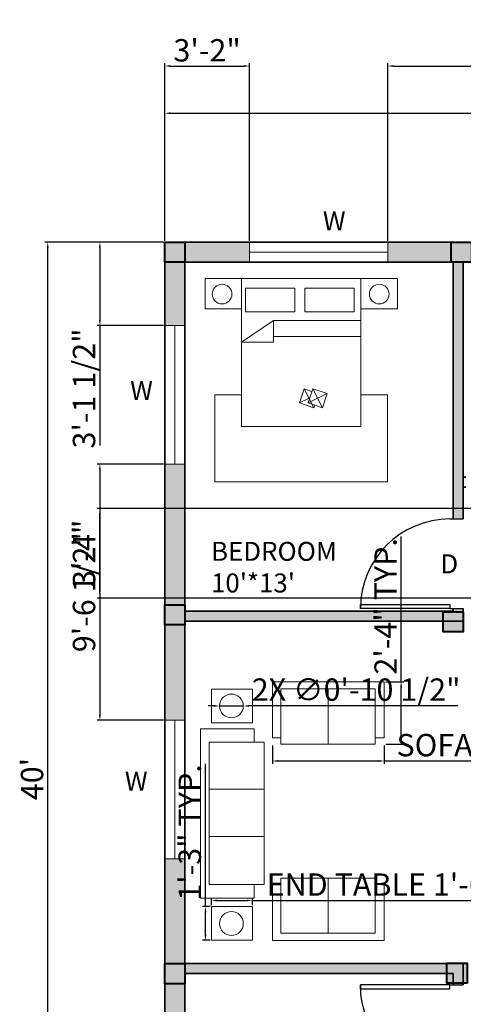
# Model space of a CAD drawing. Units: inches. Extents: x 1801 to 2333, y 2020 to 2714.
# Tile 2 of 4: x 1801 to 1999, y 2274 to 2714. Entities that reach past the tile are written whole.
import ezdxf

# ---------------------------------------------------------------- set-up
doc = ezdxf.new("R2010")
doc.units = ezdxf.units.IN
for name, color, linetype, lineweight in [('A-ANNO-DIMS', 2, 'Continuous', 18), ('A-ANNO-TEXT', 200, 'Continuous', 18), ('A-AREA-IDEN', 200, 'Continuous', 25), ('A-COLS', 7, 'Continuous', 40), ('A-COLS-PATT', 250, 'Continuous', 13), ('A-DOOR', 4, 'Continuous', 25), ('A-FURN', 8, 'Continuous', 18), ('A-WALL-PATT', 252, 'Continuous', 13), ('WALL', 150, 'Continuous', 35), ('WINDOW', 130, 'Continuous', 18)]:
    doc.layers.add(name, color=color, linetype=linetype, lineweight=lineweight)
doc.styles.get("Standard").update_dxf_attribs({"font": 'arial.ttf'})
doc.dimstyles.new('ISO-25', dxfattribs={"dimtxt": 10, "dimasz": 2.5, "dimexe": 1.25, "dimexo": 0.625, "dimtad": 1, "dimdec": 0, "dimlunit": 4, "dimtxsty": 'Standard', "dimcen": 2.5, "dimadec": 0, "dimazin": 0, "dimtfac": 1, "dimtdec": 0, "dimtmove": 0, "dimatfit": 3, "dimfxl": 1, "dimarcsym": 0})

# ---------------------------------------------------------------- blocks, each defined once
blk = doc.blocks.new('*U2')
for p, q in [((0, 0), (0, -6)), ((40, 0), (40, -6))]:
    blk.add_line(p, q)
blk.add_lwpolyline([(0, 0), (0, 40), (1.75, 40), (1.75, 0)], close=True)
blk.add_arc((0, 0), 40, 0, 90)
blk = doc.blocks.new('*D7')
at = {"layer": 'A-ANNO-DIMS', "color": 0, "lineweight": -2, "transparency": 16777216}
for p, q in [((1865.69, 2614.97), (1865.69, 2673.24)), ((1868.19, 2671.99), (2247.19, 2671.99)), ((2249.69, 2614.97), (2249.69, 2673.24))]:
    blk.add_line(p, q, dxfattribs=at)
at = {"layer": 'A-ANNO-DIMS', "color": 0, "transparency": 16777216}
for points in [[(1868.19, 2672.4), (1868.19, 2671.57), (1865.69, 2671.99)], [(2247.19, 2672.4), (2247.19, 2671.57), (2249.69, 2671.99)]]:
    blk.add_solid(points, dxfattribs=at)
at = {"layer": 'Defpoints', "color": 0, "transparency": 16777216}
for p in [(2249.69, 2671.99), (1865.69, 2614.35), (2249.69, 2614.35)]:
    blk.add_point(p, dxfattribs=at)
at = {"layer": 'A-ANNO-DIMS', "color": 0, "transparency": 16777216, "insert": (2057.69, 2677.72), "char_height": 10, "attachment_point": 5}
blk.add_mtext("32'", dxfattribs=at)
blk = doc.blocks.new('*D8')
at = {"layer": 'A-ANNO-DIMS', "color": 0, "lineweight": -2, "transparency": 16777216}
for p, q in [((1865.06, 2614.35), (1812.13, 2614.35)), ((1813.38, 2136.85), (1813.38, 2611.85)), ((1865.06, 2134.35), (1812.13, 2134.35))]:
    blk.add_line(p, q, dxfattribs=at)
at = {"layer": 'A-ANNO-DIMS', "color": 0, "transparency": 16777216}
for points in [[(1812.96, 2611.85), (1813.79, 2611.85), (1813.38, 2614.35)], [(1812.96, 2136.85), (1813.79, 2136.85), (1813.38, 2134.35)]]:
    blk.add_solid(points, dxfattribs=at)
at = {"layer": 'Defpoints', "color": 0, "transparency": 16777216}
for p in [(1813.38, 2614.35), (1865.69, 2614.35), (1865.69, 2134.35)]:
    blk.add_point(p, dxfattribs=at)
at = {"layer": 'A-ANNO-DIMS', "color": 0, "transparency": 16777216, "insert": (1807.65, 2374.35), "char_height": 10, "attachment_point": 5, "rotation": 90}
blk.add_mtext("40'", dxfattribs=at)
blk = doc.blocks.new('BED-DOUBLE-WITH-NIGHTSTANDS')
for p, q in [((30.54, 72.05), (16.34, 62.37)), ((69.61, 72.05), (30.54, 72.05)), ((30.54, 62.37), (30.54, 72.05)), ((16.34, 62.37), (30.54, 62.37)), ((30.54, 64.89), (69.61, 64.89)), ((44.26, 41.5), (48.62, 33.08)), ((48.1, 41.5), (52.46, 33.08)), ((16.34, 38.79), (4.34, 38.79)), ((4.34, 38.79), (4.34, 0)), ((42.19, 35.19), (46.77, 37.46)), ((46.03, 35.19), (54.53, 39.39)), ((69.61, 38.79), (81.61, 38.79)), ((81.61, 38.79), (81.61, 0)), ((4.34, 0), (81.61, 0))]:
    blk.add_line(p, q)
for points in [[(0, 90.88), (16.34, 90.88), (16.34, 77.31), (0, 77.31)], [(16.34, 90.88), (69.61, 90.88), (69.61, 24.72), (16.34, 24.72)], [(69.61, 90.88), (85.96, 90.88), (85.96, 77.31), (69.61, 77.31)], [(18.06, 86.51), (40.1, 86.51), (40.1, 75.9), (18.06, 75.9)], [(44.61, 86.51), (66.65, 86.51), (66.65, 75.9), (44.61, 75.9)], [(46.03, 35.19), (48.1, 41.5), (54.53, 39.39), (52.46, 33.08)]]:
    blk.add_lwpolyline(points, close=True)
blk.add_lwpolyline([(48.99, 34.22), (48.62, 33.08), (42.19, 35.19), (44.26, 41.5), (47.73, 40.36)])
for centre in [(7.61, 83.86), (77.85, 83.86)]:
    blk.add_circle(centre, 4.4)
blk = doc.blocks.new('SOFA-TWO-SEAT')
for p, q in [((50.06, 27.92), (0, 27.92)), ((0, 27.92), (0, 2.87)), ((50.06, 2.87), (50.06, 27.92)), ((3.85, 24.67), (3.85, 0)), ((24.92, 24.67), (24.92, 0)), ((0, 2.87), (3.85, 2.87)), ((45.99, 2.87), (50.06, 2.87))]:
    blk.add_line(p, q)
blk.add_lwpolyline([(3.85, 0), (45.99, 0), (45.99, 24.67), (3.85, 24.67)])
blk = doc.blocks.new('TABLE-END-WITH-LAMP')
blk.add_lwpolyline([(0, 15.04), (18.33, 15.04), (18.33, 0), (0, 0)], close=True)
blk.add_circle((8.87, 7.48), 5.32)
blk = doc.blocks.new('WIN-STANDARD')
blk.add_line((0, 4.5), (61.87, 4.5))
blk.add_lwpolyline([(0, 9), (61.87, 9), (61.87, 0), (0, 0)], close=True)
blk = doc.blocks.new('COLUMN-9X9')
blk.add_lwpolyline([(0, 9), (9, 9), (9, 0), (0, 0)], close=True)
blk = doc.blocks.new('*D26')
at = {"layer": 'A-ANNO-DIMS', "color": 0, "lineweight": -2, "transparency": 16777216}
for p, q in [((1913.81, 2389.31), (1913.81, 2381.17)), ((1963.87, 2389.31), (1963.87, 2381.17)), ((1916.31, 2382.42), (1961.37, 2382.42)), ((1963.87, 2382.42), (2070.44, 2382.42))]:
    blk.add_line(p, q, dxfattribs=at)
at = {"layer": 'A-ANNO-DIMS', "color": 0, "transparency": 16777216}
for points in [[(1916.31, 2382.84), (1916.31, 2382.01), (1913.81, 2382.42)], [(1961.37, 2382.84), (1961.37, 2382.01), (1963.87, 2382.42)]]:
    blk.add_solid(points, dxfattribs=at)
at = {"layer": 'Defpoints', "color": 0, "transparency": 16777216}
for p in [(1913.81, 2389.93), (1963.87, 2389.93), (1963.87, 2382.42)]:
    blk.add_point(p, dxfattribs=at)
at = {"layer": 'A-ANNO-DIMS', "color": 0, "transparency": 16777216, "insert": (2018.41, 2388.22), "char_height": 10, "attachment_point": 5}
blk.add_mtext('SOFA 4\'-2" TYP.', dxfattribs=at)
blk = doc.blocks.new('*D27')
at = {"layer": 'A-ANNO-DIMS', "color": 0, "lineweight": -2, "transparency": 16777216}
for p, q in [((1971.38, 2417.85), (1971.38, 2482.73)), ((1964.49, 2417.85), (1972.63, 2417.85)), ((1971.38, 2392.43), (1971.38, 2415.35)), ((1964.49, 2389.93), (1972.63, 2389.93))]:
    blk.add_line(p, q, dxfattribs=at)
at = {"layer": 'A-ANNO-DIMS', "color": 0, "transparency": 16777216}
for points in [[(1970.96, 2415.35), (1971.79, 2415.35), (1971.38, 2417.85)], [(1970.96, 2392.43), (1971.79, 2392.43), (1971.38, 2389.93)]]:
    blk.add_solid(points, dxfattribs=at)
at = {"layer": 'Defpoints', "color": 0, "transparency": 16777216}
for p in [(1963.87, 2417.85), (1971.38, 2417.85), (1963.87, 2389.93)]:
    blk.add_point(p, dxfattribs=at)
at = {"layer": 'A-ANNO-DIMS', "color": 0, "transparency": 16777216, "insert": (1965.73, 2451.54), "char_height": 10, "attachment_point": 5, "rotation": 90}
blk.add_mtext('2\'-4" TYP.', dxfattribs=at)
blk = doc.blocks.new('*D28')
at = {"layer": 'A-ANNO-DIMS', "color": 0, "lineweight": -2, "transparency": 16777216}
for p, q in [((1886.64, 2317.95), (1886.64, 2321.32)), ((1889.14, 2320.07), (1902.46, 2320.07)), ((1904.96, 2317.95), (1904.96, 2321.32)), ((1904.96, 2320.07), (2073.96, 2320.07))]:
    blk.add_line(p, q, dxfattribs=at)
at = {"layer": 'A-ANNO-DIMS', "color": 0, "transparency": 16777216}
for points in [[(1889.14, 2320.49), (1889.14, 2319.65), (1886.64, 2320.07)], [(1902.46, 2320.49), (1902.46, 2319.65), (1904.96, 2320.07)]]:
    blk.add_solid(points, dxfattribs=at)
at = {"layer": 'Defpoints', "color": 0, "transparency": 16777216}
for p in [(1904.96, 2320.07), (1886.64, 2317.32), (1904.96, 2317.32)]:
    blk.add_point(p, dxfattribs=at)
at = {"layer": 'A-ANNO-DIMS', "color": 0, "transparency": 16777216, "insert": (1990.71, 2325.87), "char_height": 10, "attachment_point": 5}
blk.add_mtext('END TABLE 1\'-6 1/2" TYP.', dxfattribs=at)
blk = doc.blocks.new('*D29')
at = {"layer": 'A-ANNO-DIMS', "color": 0, "lineweight": -2, "transparency": 16777216}
for p, q in [((1883.89, 2317.32), (1883.89, 2381.09)), ((1886.01, 2317.32), (1882.64, 2317.32)), ((1883.89, 2304.78), (1883.89, 2314.82)), ((1886.01, 2302.28), (1882.64, 2302.28))]:
    blk.add_line(p, q, dxfattribs=at)
at = {"layer": 'A-ANNO-DIMS', "color": 0, "transparency": 16777216}
for points in [[(1883.47, 2314.82), (1884.3, 2314.82), (1883.89, 2317.32)], [(1883.47, 2304.78), (1884.3, 2304.78), (1883.89, 2302.28)]]:
    blk.add_solid(points, dxfattribs=at)
at = {"layer": 'Defpoints', "color": 0, "transparency": 16777216}
for p in [(1883.89, 2317.32), (1886.64, 2317.32), (1886.64, 2302.28)]:
    blk.add_point(p, dxfattribs=at)
at = {"layer": 'A-ANNO-DIMS', "color": 0, "transparency": 16777216, "insert": (1878.15, 2350.45), "char_height": 10, "attachment_point": 5, "rotation": 90}
blk.add_mtext('1\'-3" TYP.', dxfattribs=at)
blk = doc.blocks.new('*D30')
at = {"layer": 'A-ANNO-DIMS', "color": 0, "lineweight": -2, "transparency": 16777216}
for p, q in [((1865.69, 2614.97), (1865.69, 2694.33)), ((1903.59, 2614.97), (1903.59, 2694.33)), ((1868.19, 2693.08), (1901.09, 2693.08))]:
    blk.add_line(p, q, dxfattribs=at)
at = {"layer": 'A-ANNO-DIMS', "color": 0, "transparency": 16777216}
for points in [[(1868.19, 2693.5), (1868.19, 2692.66), (1865.69, 2693.08)], [(1901.09, 2693.5), (1901.09, 2692.66), (1903.59, 2693.08)]]:
    blk.add_solid(points, dxfattribs=at)
at = {"layer": 'Defpoints', "color": 0, "transparency": 16777216}
for p in [(1903.59, 2693.08), (1865.69, 2614.35), (1903.59, 2614.35)]:
    blk.add_point(p, dxfattribs=at)
at = {"layer": 'A-ANNO-DIMS', "color": 0, "transparency": 16777216, "insert": (1884.64, 2698.81), "char_height": 10, "attachment_point": 5}
blk.add_mtext('3\'-2"', dxfattribs=at)
blk = doc.blocks.new('*D31')
at = {"layer": 'A-ANNO-DIMS', "color": 0, "lineweight": -2, "transparency": 16777216}
for p, q in [((1965.46, 2614.97), (1965.46, 2694.33)), ((2008.88, 2614.97), (2008.88, 2694.33)), ((1967.96, 2693.08), (2006.38, 2693.08)), ((2008.88, 2693.08), (2062.5, 2693.08))]:
    blk.add_line(p, q, dxfattribs=at)
at = {"layer": 'A-ANNO-DIMS', "color": 0, "transparency": 16777216}
for points in [[(1967.96, 2693.5), (1967.96, 2692.66), (1965.46, 2693.08)], [(2006.38, 2693.5), (2006.38, 2692.66), (2008.88, 2693.08)]]:
    blk.add_solid(points, dxfattribs=at)
at = {"layer": 'Defpoints', "color": 0, "transparency": 16777216}
for p in [(2008.88, 2693.08), (1965.46, 2614.35), (2008.88, 2614.35)]:
    blk.add_point(p, dxfattribs=at)
at = {"layer": 'A-ANNO-DIMS', "color": 0, "transparency": 16777216, "insert": (2036.94, 2698.88), "char_height": 10, "attachment_point": 5}
blk.add_mtext('3\'-7 1/2"', dxfattribs=at)
blk = doc.blocks.new('*D34')
at = {"layer": 'A-ANNO-DIMS', "color": 0, "lineweight": -2, "transparency": 16777216}
for p, q in [((1865.06, 2614.35), (1835.44, 2614.35)), ((1836.69, 2611.85), (1836.69, 2579.52)), ((1865.06, 2577.02), (1835.44, 2577.02)), ((1836.69, 2577.02), (1836.69, 2523.39))]:
    blk.add_line(p, q, dxfattribs=at)
at = {"layer": 'A-ANNO-DIMS', "color": 0, "transparency": 16777216}
for points in [[(1836.27, 2611.85), (1837.11, 2611.85), (1836.69, 2614.35)], [(1836.27, 2579.52), (1837.11, 2579.52), (1836.69, 2577.02)]]:
    blk.add_solid(points, dxfattribs=at)
at = {"layer": 'Defpoints', "color": 0, "transparency": 16777216}
for p in [(1865.69, 2614.35), (1836.69, 2577.02), (1865.69, 2577.02)]:
    blk.add_point(p, dxfattribs=at)
at = {"layer": 'A-ANNO-DIMS', "color": 0, "transparency": 16777216, "insert": (1830.89, 2548.95), "char_height": 10, "attachment_point": 5, "rotation": 90}
blk.add_mtext('3\'-1 1/2"', dxfattribs=at)
blk = doc.blocks.new('*D35')
at = {"layer": 'A-ANNO-DIMS', "color": 0, "lineweight": -2, "transparency": 16777216}
for p, q in [((1865.06, 2515.15), (1835.44, 2515.15)), ((1836.69, 2512.65), (1836.69, 2403.11)), ((1865.06, 2400.61), (1835.44, 2400.61))]:
    blk.add_line(p, q, dxfattribs=at)
at = {"layer": 'A-ANNO-DIMS', "color": 0, "transparency": 16777216}
for points in [[(1836.27, 2512.65), (1837.11, 2512.65), (1836.69, 2515.15)], [(1836.27, 2403.11), (1837.11, 2403.11), (1836.69, 2400.61)]]:
    blk.add_solid(points, dxfattribs=at)
at = {"layer": 'Defpoints', "color": 0, "transparency": 16777216}
for p in [(1865.69, 2515.15), (1836.69, 2400.61), (1865.69, 2400.61)]:
    blk.add_point(p, dxfattribs=at)
at = {"layer": 'A-ANNO-DIMS', "color": 0, "transparency": 16777216, "insert": (1830.89, 2457.88), "char_height": 10, "attachment_point": 5, "rotation": 90}
blk.add_mtext('9\'-6 1/2"', dxfattribs=at)
blk = doc.blocks.new('*D48')
at = {"layer": 'A-ANNO-DIMS', "color": 0, "lineweight": -2, "transparency": 16777216}
for p, q in [((2115.56, 2495.25), (1835.44, 2495.25)), ((1836.69, 2457.75), (1836.69, 2492.75)), ((2115.56, 2455.25), (1835.44, 2455.25))]:
    blk.add_line(p, q, dxfattribs=at)
at = {"layer": 'A-ANNO-DIMS', "color": 0, "transparency": 16777216}
for points in [[(1836.27, 2492.75), (1837.11, 2492.75), (1836.69, 2495.25)], [(1836.27, 2457.75), (1837.11, 2457.75), (1836.69, 2455.25)]]:
    blk.add_solid(points, dxfattribs=at)
at = {"layer": 'Defpoints', "color": 0, "transparency": 16777216}
for p in [(1836.69, 2495.25), (2116.19, 2495.25), (2116.19, 2455.25)]:
    blk.add_point(p, dxfattribs=at)
at = {"layer": 'A-ANNO-DIMS', "color": 0, "transparency": 16777216, "insert": (1830.95, 2475.25), "char_height": 10, "attachment_point": 5, "rotation": 90}
blk.add_mtext('3\'-4"', dxfattribs=at)
blk = doc.blocks.new('*D58')
at = {"layer": 'A-ANNO-DIMS', "color": 0, "lineweight": -2, "transparency": 16777216}
for p, q in [((1887.68, 2407.01), (1885.18, 2407.01)), ((1890.18, 2407.01), (1900.83, 2407.01)), ((1996.73, 2407.01), (1903.33, 2407.01))]:
    blk.add_line(p, q, dxfattribs=at)
at = {"layer": 'A-ANNO-DIMS', "color": 0, "transparency": 16777216}
for points in [[(1887.68, 2407.43), (1887.68, 2406.6), (1890.18, 2407.01)], [(1903.33, 2407.43), (1903.33, 2406.6), (1900.83, 2407.01)]]:
    blk.add_solid(points, dxfattribs=at)
at = {"layer": 'Defpoints', "color": 0, "transparency": 16777216}
for p in [(1890.18, 2407.01), (1900.83, 2407.01)]:
    blk.add_point(p, dxfattribs=at)
at = {"layer": 'A-ANNO-DIMS', "color": 0, "transparency": 16777216, "insert": (1951.28, 2413.02), "char_height": 10, "attachment_point": 5, "rotation": 359.9978}
blk.add_mtext('2X ∅0\'-10 1/2"', dxfattribs=at)

msp = doc.modelspace()

# ---------------------------------------------------------------- hatches: boundary and pattern name
at = {"layer": 'A-COLS-PATT'}
h = msp.add_hatch(color=256, dxfattribs=at)
h.dxf.hatch_style = 1
h.paths.add_polyline_path([(1874.69, 2614.35), (1865.69, 2614.35), (1865.69, 2605.35), (1874.69, 2605.35)])
h.paths.add_polyline_path([(2002.83, 2614.35), (1993.83, 2614.35), (1993.83, 2605.35), (2002.83, 2605.35)])
h.paths.add_polyline_path([(2117.06, 2614.35), (2108.06, 2614.35), (2108.06, 2605.35), (2117.06, 2605.35)])
h.paths.add_polyline_path([(2249.69, 2614.35), (2240.69, 2614.35), (2240.69, 2605.35), (2249.69, 2605.35)])
h.paths.add_polyline_path([(1874.69, 2452.27), (1865.69, 2452.27), (1865.69, 2443.27), (1874.69, 2443.27)])
h.paths.add_polyline_path([(1999.19, 2449.12), (1990.19, 2449.12), (1990.19, 2444.85), (1999.19, 2444.85)])
h.paths.add_polyline_path([(1999.19, 2444.85), (1990.19, 2444.85), (1990.19, 2440.12), (1999.19, 2440.12)])
h.paths.add_polyline_path([(2120.9, 2449.35), (2116.19, 2449.35), (2116.19, 2453.56), (2111.9, 2453.56), (2111.9, 2444.85), (2120.9, 2444.85)])
h.paths.add_polyline_path([(2120.9, 2453.56), (2116.19, 2453.56), (2116.19, 2449.35), (2120.9, 2449.35)], flags=17)
h.paths.add_polyline_path([(2249.69, 2451.04), (2240.69, 2451.04), (2240.69, 2442.04), (2249.69, 2442.04)])
h.paths.add_polyline_path([(2249.69, 2330.92), (2240.69, 2330.92), (2240.69, 2321.92), (2249.69, 2321.92)])
h.paths.add_polyline_path([(2115.69, 2329.7), (2111.19, 2329.7), (2111.19, 2324.35), (2115.69, 2324.35)])
h.paths.add_polyline_path([(2115.69, 2324.35), (2111.19, 2324.35), (2111.19, 2320.7), (2115.69, 2320.7)])
h.paths.add_polyline_path([(2111.19, 2329.7), (2106.69, 2329.7), (2106.69, 2320.7), (2111.19, 2320.7), (2111.19, 2324.35)])
h.paths.add_polyline_path([(1999.19, 2291.85), (1991.86, 2291.85), (1991.86, 2287.35), (1994.69, 2287.35), (1994.69, 2283.08), (1999.19, 2283.08)], flags=17)
h.paths.add_polyline_path([(2000.86, 2292.08), (1991.86, 2292.08), (1991.86, 2291.85), (1999.19, 2291.85), (1999.19, 2283.08), (2000.86, 2283.08)])
h.paths.add_polyline_path([(1994.69, 2287.35), (1991.86, 2287.35), (1991.86, 2283.08), (1994.69, 2283.08)], flags=16)
h.paths.add_polyline_path([(1874.69, 2143.35), (1865.69, 2143.35), (1865.69, 2134.35), (1874.69, 2134.35)])
h.paths.add_polyline_path([(1999.19, 2143.35), (1990.19, 2143.35), (1990.19, 2134.35), (1999.19, 2134.35)])
h.paths.add_polyline_path([(2118.63, 2143.35), (2109.63, 2143.35), (2109.63, 2134.35), (2118.63, 2134.35)])
h.paths.add_polyline_path([(2249.69, 2143.35), (2240.69, 2143.35), (2240.69, 2134.35), (2249.69, 2134.35)])
h = msp.add_hatch(color=256, dxfattribs=at)
h.dxf.hatch_style = 1
h.paths.add_polyline_path([(1874.69, 2291.85), (1865.69, 2291.85), (1865.69, 2282.85), (1874.69, 2282.85)])
at = {"layer": 'A-WALL-PATT'}
h = msp.add_hatch(color=256, dxfattribs=at)
h.dxf.hatch_style = 1
h.paths.add_polyline_path([(2067.79, 2614.35), (2044.01, 2614.35), (2044.01, 2605.35), (2053.19, 2605.35), (2067.79, 2605.35)])
h.paths.add_polyline_path([(2057.69, 2605.35), (2053.19, 2605.35), (2053.19, 2509.35), (2040.35, 2509.35), (2030.72, 2509.35), (2030.72, 2504.85), (2040.35, 2504.85), (2057.69, 2504.85), (2111.69, 2504.85), (2111.69, 2509.35), (2057.69, 2509.35)])
h.paths.add_polyline_path([(1999.19, 2605.35), (1994.69, 2605.35), (1994.69, 2490.6), (1999.19, 2490.6)])
h.paths.add_polyline_path([(2116.19, 2605.35), (2111.69, 2605.35), (2111.69, 2550.35), (2111.69, 2535.67, -0.006913), (2112.39, 2535.68), (2116.19, 2535.68), (2116.19, 2551.5)])
h.paths.add_polyline_path([(2116.19, 2510.35), (2112.39, 2510.35), (2111.69, 2510.35), (2111.69, 2495.25), (2116.19, 2495.25)])
h.paths.add_polyline_path([(2115.69, 2273.91), (2111.19, 2273.91), (2111.19, 2143.35), (2115.69, 2143.35)], flags=17)
h.paths.add_polyline_path([(2118.63, 2143.35), (2118.63, 2134.35), (2159.47, 2134.35), (2159.47, 2143.35)])
h.paths.add_polyline_path([(2109.63, 2134.35), (2109.63, 2143.35), (2082.87, 2143.35), (2082.87, 2134.35)])
h.paths.add_polyline_path([(1999.19, 2143.35), (1999.19, 2134.35), (2021.01, 2134.35), (2021.01, 2143.35)])
h.paths.add_polyline_path([(1990.19, 2134.35), (1990.19, 2143.35), (1965.15, 2143.35), (1965.15, 2134.35)])
h.paths.add_polyline_path([(1903.28, 2143.35), (1874.69, 2143.35), (1874.69, 2134.35), (1903.28, 2134.35)])
h.paths.add_polyline_path([(1865.69, 2143.35), (1874.69, 2143.35), (1874.69, 2183.28), (1865.69, 2183.28)])
h.paths.add_polyline_path([(1991.86, 2287.35), (1991.86, 2291.85), (1874.69, 2291.85), (1874.69, 2287.35)])
h.paths.add_polyline_path([(1999.19, 2283.08), (1994.69, 2283.08), (1994.69, 2282.32), (1999.19, 2282.32)])
h.paths.add_polyline_path([(1865.69, 2452.27), (1874.69, 2452.27), (1874.69, 2515.15), (1865.69, 2515.15)])
h.paths.add_polyline_path([(1874.69, 2443.27), (1865.69, 2443.27), (1865.69, 2400.61), (1874.69, 2400.61)])
h.paths.add_polyline_path([(2120.9, 2449.35), (2120.9, 2444.85), (2240.69, 2444.85), (2240.69, 2449.35)])
h.paths.add_polyline_path([(2111.9, 2453.56), (2116.19, 2453.56), (2116.19, 2455.25), (2111.69, 2455.25), (2111.69, 2444.85), (2111.9, 2444.85)])
h.paths.add_polyline_path([(1874.69, 2605.35), (1865.69, 2605.35), (1865.69, 2577.02), (1874.69, 2577.02)])
h.paths.add_polyline_path([(1874.69, 2614.35), (1874.69, 2605.35), (1903.59, 2605.35), (1903.59, 2614.35)])
h = msp.add_hatch(color=256, dxfattribs=at)
h.dxf.hatch_style = 1
h.paths.add_polyline_path([(2118.63, 2143.35), (2118.63, 2134.35), (2159.47, 2134.35), (2159.47, 2143.35)])
h.paths.add_polyline_path([(2109.63, 2134.35), (2109.63, 2143.35), (2082.87, 2143.35), (2082.87, 2134.35)])
h.paths.add_polyline_path([(1999.19, 2143.35), (1999.19, 2134.35), (2021.01, 2134.35), (2021.01, 2143.35)])
h.paths.add_polyline_path([(1990.19, 2134.35), (1990.19, 2143.35), (1965.15, 2143.35), (1965.15, 2134.35)])
h.paths.add_polyline_path([(1874.69, 2143.35), (1874.69, 2134.35), (1903.28, 2134.35), (1903.28, 2143.35)])
h.paths.add_polyline_path([(1865.69, 2143.35), (1874.69, 2143.35), (1874.69, 2183.28), (1865.69, 2183.28)])
h.paths.add_polyline_path([(1874.69, 2443.27), (1865.69, 2443.27), (1865.69, 2400.61), (1874.69, 2400.61)])
h.paths.add_polyline_path([(1865.69, 2452.27), (1874.69, 2452.27), (1874.69, 2515.15), (1865.69, 2515.15)])
h.paths.add_polyline_path([(1874.69, 2577.02), (1874.69, 2605.35), (1865.69, 2605.35), (1865.69, 2577.02)])
h.paths.add_polyline_path([(1874.69, 2614.35), (1874.69, 2605.35), (1903.59, 2605.35), (1903.59, 2614.35)])
h.paths.add_polyline_path([(2240.69, 2605.35), (2240.69, 2614.35), (2203.01, 2614.35), (2203.01, 2605.35)])
h.paths.add_polyline_path([(2249.69, 2605.35), (2240.69, 2605.35), (2240.69, 2567.46), (2249.69, 2567.46)])
h = msp.add_hatch(color=256, dxfattribs=at)
h.dxf.hatch_style = 1
h.paths.add_polyline_path([(2249.69, 2505.59), (2240.69, 2505.59), (2240.69, 2451.04), (2249.69, 2451.04)])
h.paths.add_polyline_path([(2249.69, 2442.04), (2240.69, 2442.04), (2240.69, 2424.01), (2249.69, 2424.01)])
h.paths.add_polyline_path([(2249.69, 2362.14), (2240.69, 2362.14), (2240.69, 2330.92), (2249.69, 2330.92)])
h.paths.add_polyline_path([(2249.69, 2321.92), (2240.69, 2321.92), (2240.69, 2143.35), (2249.69, 2143.35)])
h.paths.add_polyline_path([(2240.69, 2143.35), (2214.05, 2143.35), (2214.05, 2134.35), (2240.69, 2134.35)])
h.paths.add_polyline_path([(1874.69, 2282.85), (1865.69, 2282.85), (1865.69, 2245.15), (1874.69, 2245.15)])
h.paths.add_polyline_path([(1874.69, 2338.74), (1865.69, 2338.74), (1865.69, 2291.85), (1874.69, 2291.85)])
h.paths.add_polyline_path([(1990.19, 2449.12), (1999.19, 2449.12), (1999.19, 2450.6), (1994.69, 2450.6), (1994.69, 2449.35), (1874.69, 2449.35), (1874.69, 2444.85), (1990.19, 2444.85)])
h.paths.add_polyline_path([(2141.14, 2614.35), (2117.06, 2614.35), (2117.06, 2605.35), (2141.14, 2605.35)])
h.paths.add_polyline_path([(2108.06, 2614.35), (2102.92, 2614.35), (2102.92, 2605.35), (2108.06, 2605.35)])
h.paths.add_polyline_path([(1993.83, 2614.35), (1965.46, 2614.35), (1965.46, 2605.35), (1993.83, 2605.35)])
h.paths.add_polyline_path([(2008.88, 2614.35), (2002.83, 2614.35), (2002.83, 2605.35), (2008.88, 2605.35)])
h.paths.add_polyline_path([(2107.38, 2466.24), (2120.18, 2466.24), (2120.18, 2483.72), (2107.38, 2483.72)], flags=9)
h.paths.add_polyline_path([(2104.14, 2515.21), (2116.94, 2515.21), (2116.94, 2532.69), (2104.14, 2532.69)], flags=9)
h.paths.add_polyline_path([(2007.5, 2499.97), (2020.3, 2499.97), (2020.3, 2517.44), (2007.5, 2517.44)], flags=9)
h.paths.add_polyline_path([(1985.91, 2461.68), (1998.7, 2461.68), (1998.7, 2479.15), (1985.91, 2479.15)], flags=9)
h.paths.add_polyline_path([(2109.98, 2348.28), (2122.78, 2348.28), (2122.78, 2365.76), (2109.98, 2365.76)], flags=9)
h.paths.add_polyline_path([(1977.13, 2255.51), (1989.93, 2255.51), (1989.93, 2272.99), (1977.13, 2272.99)], flags=9)
h.paths.add_polyline_path([(2063.1, 2540.71), (2101.48, 2540.71), (2101.48, 2560.24), (2063.1, 2560.24)], flags=9)
h.paths.add_polyline_path([(1995.81, 2316.5), (2071.83, 2316.5), (2071.83, 2348.15), (1995.81, 2348.15)], flags=9)
h.paths.add_polyline_path([(2138.31, 2394.68), (2194.97, 2394.68), (2194.97, 2426.33), (2138.31, 2426.33)], flags=9)
h.paths.add_polyline_path([(2163.82, 2472.81), (2229.7, 2472.81), (2229.7, 2504.45), (2163.82, 2504.45)], flags=9)
h.paths.add_polyline_path([(2007.01, 2540.94), (2045.38, 2540.94), (2045.38, 2560.47), (2007.01, 2560.47)], flags=9)
h.paths.add_polyline_path([(1882.98, 2452.95), (1948.86, 2452.95), (1948.86, 2484.59), (1882.98, 2484.59)], flags=9)

# ---------------------------------------------------------------- linework, layer by layer
at = {"layer": 'A-FURN'}
for p, q in [((1881.62, 2321.14), (1881.62, 2396.72)), ((1881.62, 2396.72), (1905.74, 2396.72)), ((1905.74, 2396.72), (1905.74, 2390.82)), ((1885.5, 2369.75), (1910.17, 2369.75)), ((1885.5, 2348.68), (1910.17, 2348.68)), ((1905.74, 2327.28), (1905.74, 2321.14)), ((1905.74, 2321.14), (1881.62, 2321.14))]:
    msp.add_line(p, q, dxfattribs=at)
msp.add_lwpolyline([(1885.5, 2327.28), (1910.17, 2327.28), (1910.17, 2390.82), (1885.5, 2390.82)], close=True, dxfattribs=at)
at = {"layer": 'WALL'}
for p, q in [((1874.69, 2605.35), (1994.69, 2605.35)), ((1994.69, 2605.35), (1994.69, 2490.6)), ((1999.19, 2605.35), (1999.19, 2490.6)), ((1999.19, 2605.35), (2053.19, 2605.35)), ((2000.35, 2509.35), (1999.19, 2509.35)), ((2000.35, 2504.85), (1999.19, 2504.85)), ((1994.69, 2449.35), (1874.69, 2449.35)), ((1994.69, 2450.6), (1994.69, 2449.35)), ((1999.19, 2450.6), (1999.19, 2444.85)), ((1999.19, 2444.85), (1874.69, 2444.85)), ((1999.19, 2291.85), (1874.69, 2291.85)), ((1999.19, 2282.32), (1999.19, 2291.85)), ((1994.69, 2287.35), (1874.69, 2287.35)), ((1994.69, 2282.32), (1994.69, 2287.35))]:
    msp.add_line(p, q, dxfattribs=at)
for points in [[(2214.05, 2134.35), (2249.69, 2134.35), (2249.69, 2614.35), (1865.69, 2614.35), (1865.69, 2134.35), (2159.47, 2134.35)], [(2214.05, 2143.35), (2240.69, 2143.35), (2240.69, 2605.35), (1874.69, 2605.35), (1874.69, 2143.35), (2159.47, 2143.35)]]:
    msp.add_lwpolyline(points, dxfattribs=at)

# ---------------------------------------------------------------- block references
at = {"layer": 'A-COLS'}
for p in [(1865.69, 2605.35), (1993.83, 2605.35), (1865.69, 2443.27), (1990.19, 2440.12), (1865.69, 2282.85), (1991.86, 2283.08)]:
    msp.add_blockref('COLUMN-9X9', p, dxfattribs=at)
at = {"layer": 'A-DOOR', "rotation": 90}
msp.add_blockref('*U2', (1993.19, 2450.6), dxfattribs=at)
at = {"layer": 'A-DOOR', "xscale": -1, "rotation": 90}
msp.add_blockref('*U2', (1993.19, 2282.32), dxfattribs=at)
at = {"layer": 'A-FURN'}
for name, p in [('BED-DOUBLE-WITH-NIGHTSTANDS', (1883.74, 2507.27)), ('SOFA-TWO-SEAT', (1913.81, 2389.93)), ('TABLE-END-WITH-LAMP', (1886.63, 2399.53)), ('TABLE-END-WITH-LAMP', (1886.63, 2302.28))]:
    msp.add_blockref(name, p, dxfattribs=at)
at = {"layer": 'A-FURN', "extrusion": (0, 0, -1), "zscale": -1, "rotation": 180}
msp.add_blockref('SOFA-TWO-SEAT', (-1913.81, 2330.07), dxfattribs=at)
at = {"layer": 'WINDOW'}
msp.add_blockref('WIN-STANDARD', (1903.59, 2605.35), dxfattribs=at)
for p, rotation in [((1865.69, 2577.02), 270.0000000000002), ((1865.69, 2400.61), 270.0000000000001)]:
    msp.add_blockref('WIN-STANDARD', p, dxfattribs=dict(at, rotation=rotation))

# ---------------------------------------------------------------- texts
at = {"layer": 'A-ANNO-TEXT', "char_height": 8.48, "attachment_point": 1}
for s, insert in [('W', (1936.39, 2628.09)), ('W', (1850.22, 2552.28)), ('D', (1988.94, 2474.79)), ('W', (1847.87, 2377.6))]:
    msp.add_mtext_dynamic_manual_height_columns(s, width=170.2706, gutter_width=42.4, heights=[0], dxfattribs=dict(at, insert=insert))
at = {"layer": 'A-AREA-IDEN', "insert": (1886.39, 2480.38), "char_height": 8.481, "attachment_point": 1}
msp.add_mtext_dynamic_manual_height_columns("BEDROOM\\P10'*13'", width=170.2706, gutter_width=42.4, heights=[0], dxfattribs=at)

# ---------------------------------------------------------------- dimensions: what is measured, and where the dimension line sits
at = {"layer": 'A-ANNO-DIMS'}
for base, p1, p2, override, picture, middle in [((2008.88, 2693.08), (1965.46, 2614.35), (2008.88, 2614.35), {"dimdec": 1, "dimlfac": 1, "dimrnd": 0, "dimzin": 1, "dimdsep": 46, "dimlunit": 4, "dimfrac": 2}, '*D31', (2036.94, 2698.88)), ((1903.59, 2693.08), (1865.69, 2614.35), (1903.59, 2614.35), {"dimdec": 1, "dimlfac": 1, "dimrnd": 0, "dimzin": 1, "dimdsep": 46, "dimlunit": 4, "dimfrac": 2}, '*D30', (1884.64, 2698.81)), ((2249.69, 2671.99), (1865.69, 2614.35), (2249.69, 2614.35), {"dimclrd": 0, "dimclre": 0, "dimclrt": 0}, '*D7', (2057.69, 2677.72))]:
    dim = msp.add_linear_dim(base=base, p1=p1, p2=p2, dimstyle='ISO-25', override=override, dxfattribs=at)
    dim.commit()
    dim.dimension.update_dxf_attribs({"geometry": picture, "text_midpoint": middle})
for base, p1, p2, override, picture, middle in [((1813.38, 2614.35), (1865.69, 2134.35), (1865.69, 2614.35), {"dimclrd": 0, "dimclre": 0, "dimclrt": 0}, '*D8', (1807.65, 2374.35)), ((1836.69, 2577.02), (1865.69, 2614.35), (1865.69, 2577.02), {"dimdec": 1, "dimlfac": 1, "dimrnd": 0, "dimzin": 1, "dimdsep": 46, "dimlunit": 4, "dimfrac": 2}, '*D34', (1830.89, 2548.95)), ((1836.69, 2400.61), (1865.69, 2515.15), (1865.69, 2400.61), {"dimdec": 1, "dimlfac": 1, "dimrnd": 0, "dimzin": 1, "dimdsep": 46, "dimlunit": 4, "dimfrac": 2}, '*D35', (1830.89, 2457.88)), ((1836.69, 2495.25), (2116.19, 2455.25), (2116.19, 2495.25), {"dimdec": 1, "dimlfac": 1, "dimrnd": 0, "dimzin": 1, "dimdsep": 46, "dimlunit": 4, "dimfrac": 2}, '*D48', (1830.95, 2475.25))]:
    dim = msp.add_linear_dim(base=base, p1=p1, p2=p2, angle=90, dimstyle='ISO-25', override=override, dxfattribs=at)
    dim.commit()
    dim.dimension.update_dxf_attribs({"geometry": picture, "text_midpoint": middle})
for base, p1, p2, picture, middle in [((1971.38, 2417.85), (1963.87, 2389.93), (1963.87, 2417.85), '*D27', (1965.73, 2451.54)), ((1883.89, 2317.32), (1886.64, 2302.28), (1886.64, 2317.32), '*D29', (1878.15, 2350.45))]:
    dim = msp.add_linear_dim(base=base, p1=p1, p2=p2, angle=90, text='<> TYP.', dimstyle='ISO-25', override={"dimdec": 1, "dimlfac": 1, "dimrnd": 0, "dimzin": 1, "dimdsep": 46, "dimlunit": 4, "dimfrac": 2}, dxfattribs=at)
    dim.commit()
    dim.dimension.update_dxf_attribs({"geometry": picture, "text_midpoint": middle})
dim = msp.add_diameter_dim_2p(p1=(1890.1821, 2407.0124), p2=(1900.8256, 2407.012), text='2X <>', dimstyle='ISO-25', override={"dimdec": 1, "dimlfac": 1, "dimrnd": 0, "dimzin": 1, "dimdsep": 46, "dimlunit": 4, "dimfrac": 2}, dxfattribs=at)
dim.commit()
dim.dimension.update_dxf_attribs({"geometry": '*D58', "text_midpoint": (1951.2801, 2407.01), "dimtype": 163})
for base, p1, p2, text, picture, middle in [((1963.87, 2382.42), (1913.81, 2389.93), (1963.87, 2389.93), 'SOFA <> TYP.', '*D26', (2018.41, 2388.22)), ((1904.96, 2320.07), (1886.64, 2317.32), (1904.96, 2317.32), 'END TABLE <> TYP.', '*D28', (1990.71, 2325.87))]:
    dim = msp.add_linear_dim(base=base, p1=p1, p2=p2, text=text, dimstyle='ISO-25', override={"dimdec": 1, "dimlfac": 1, "dimrnd": 0, "dimzin": 1, "dimdsep": 46, "dimlunit": 4, "dimfrac": 2}, dxfattribs=at)
    dim.commit()
    dim.dimension.update_dxf_attribs({"geometry": picture, "text_midpoint": middle})

doc.saveas('drawing.dxf')
